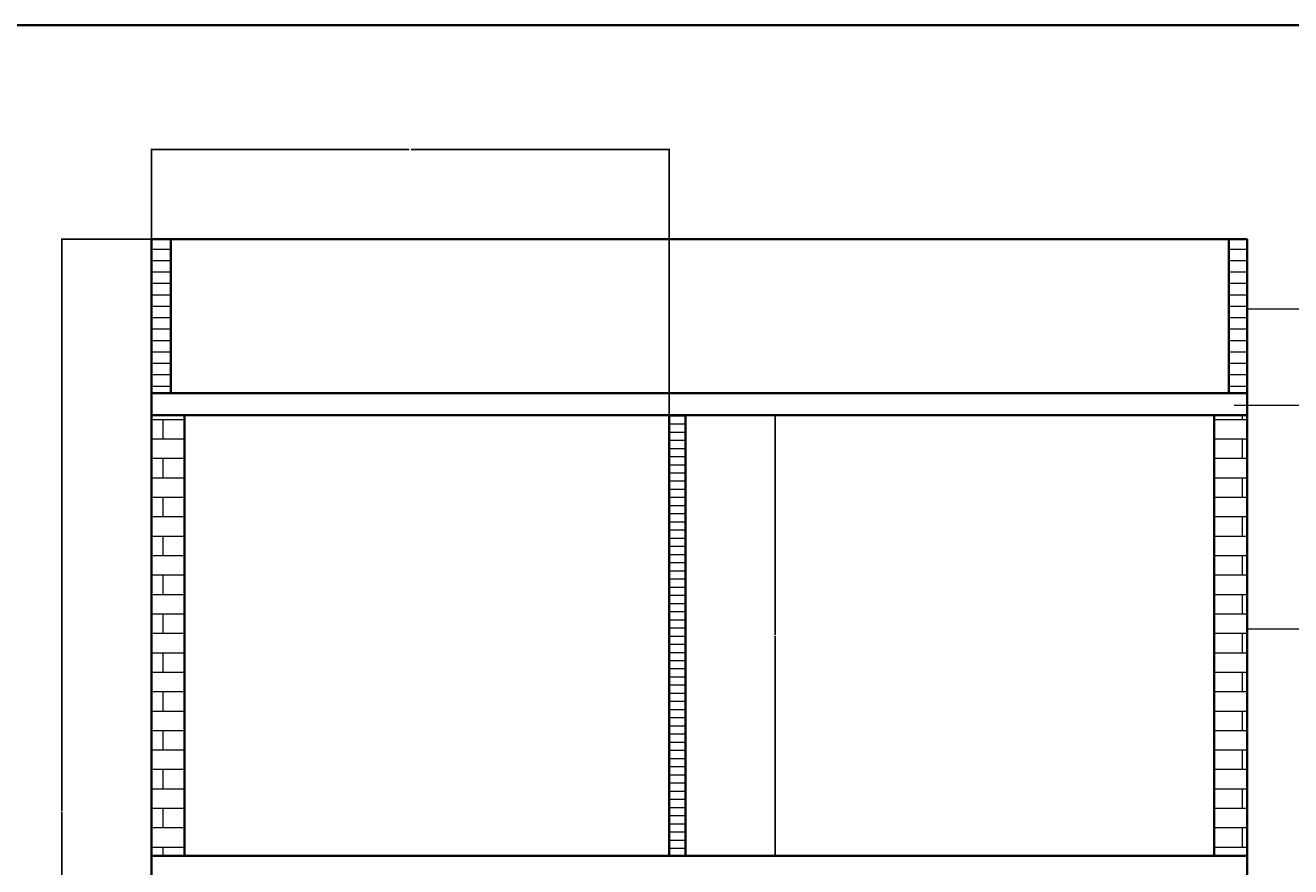
# Model space of a CAD drawing. Units: inches. Extents: x 2416 to 3391, y 1375 to 2496.
# Tile 12 of 13: x 2870 to 3215, y 2267 to 2496. Entities that reach past the tile are written whole.
import ezdxf

# ---------------------------------------------------------------- set-up
doc = ezdxf.new("R2010")
doc.units = ezdxf.units.IN
for name, color, linetype, lineweight in [('A-ANNO-DIMS', 2, 'Continuous', 18), ('A-ANNO-TEXT', 7, 'Continuous', 18), ('A-ANNO-TTLB', 7, 'Continuous', 35), ('A-SECT', 7, 'Continuous', 35), ('A-WALL-PATT', 252, 'Continuous', 13)]:
    doc.layers.add(name, color=color, linetype=linetype, lineweight=lineweight)
doc.styles.get("Standard").update_dxf_attribs({"font": 'arial.ttf'})
doc.dimstyles.get("Standard").update_dxf_attribs({"dimtxt": 0.18, "dimasz": 0.18, "dimexe": 0.18, "dimexo": 0.0625, "dimgap": 0.09, "dimtad": 0, "dimtih": 1, "dimtoh": 1, "dimdec": 4, "dimzin": 0, "dimdsep": 46, "dimtxsty": 'Standard', "dimcen": 0.09, "dimadec": 0, "dimazin": 0, "dimtfac": 1, "dimtdec": 4, "dimtofl": 0, "dimtmove": 0, "dimatfit": 3, "dimfxl": 1, "dimtolj": 1, "dimtzin": 0, "dimarcsym": 0})

# ---------------------------------------------------------------- blocks, each defined once
blk = doc.blocks.new('*D84')
at = {"layer": 'A-ANNO-DIMS', "color": 0, "lineweight": -2, "transparency": 16777216}
for p, q in [((2904.13, 2437.86), (2879.61, 2437.86)), ((2879.79, 2437.68), (2879.79, 2282.04)), ((2879.79, 2126.04), (2879.79, 2281.68)), ((2904.13, 2125.86), (2879.61, 2125.86))]:
    blk.add_line(p, q, dxfattribs=at)
at = {"layer": 'A-ANNO-DIMS', "color": 0, "transparency": 16777216}
for points in [[(2879.76, 2437.68), (2879.82, 2437.68), (2879.79, 2437.86)], [(2879.76, 2126.04), (2879.82, 2126.04), (2879.79, 2125.86)]]:
    blk.add_solid(points, dxfattribs=at)
at = {"layer": 'Defpoints', "color": 0, "transparency": 16777216}
for p in [(2879.79, 2437.86), (2904.19, 2437.86), (2904.19, 2125.86)]:
    blk.add_point(p, dxfattribs=at)
at = {"layer": 'A-ANNO-DIMS', "color": 0, "transparency": 16777216, "insert": (2879.79, 2281.86), "char_height": 0.18, "attachment_point": 5}
blk.add_mtext('\\A1;312', dxfattribs=at)
blk = doc.blocks.new('*D85')
at = {"layer": 'A-ANNO-DIMS', "color": 0, "lineweight": -2, "transparency": 16777216}
for p, q in [((2904.19, 2437.92), (2904.19, 2462.44)), ((2904.37, 2462.26), (2974.43, 2462.26)), ((3045.01, 2462.26), (2974.96, 2462.26)), ((3045.19, 2389.92), (3045.19, 2462.44))]:
    blk.add_line(p, q, dxfattribs=at)
at = {"layer": 'A-ANNO-DIMS', "color": 0, "transparency": 16777216}
for points in [[(2904.37, 2462.29), (2904.37, 2462.23), (2904.19, 2462.26)], [(3045.01, 2462.29), (3045.01, 2462.23), (3045.19, 2462.26)]]:
    blk.add_solid(points, dxfattribs=at)
at = {"layer": 'Defpoints', "color": 0, "transparency": 16777216}
for p in [(3045.19, 2462.26), (2904.19, 2437.86), (3045.19, 2389.86)]:
    blk.add_point(p, dxfattribs=at)
at = {"layer": 'A-ANNO-DIMS', "color": 0, "transparency": 16777216, "insert": (2974.69, 2462.26), "char_height": 0.18, "attachment_point": 5}
blk.add_mtext('\\A1;141', dxfattribs=at)
blk = doc.blocks.new('*D87')
at = {"layer": 'A-ANNO-DIMS', "color": 0, "lineweight": -2, "transparency": 16777216}
for p, q in [((3049.75, 2389.86), (3074.27, 2389.86)), ((3074.09, 2389.68), (3074.09, 2330.04)), ((3074.09, 2270.04), (3074.09, 2329.68)), ((3049.75, 2269.86), (3074.27, 2269.86))]:
    blk.add_line(p, q, dxfattribs=at)
at = {"layer": 'A-ANNO-DIMS', "color": 0, "transparency": 16777216}
for points in [[(3074.06, 2389.68), (3074.12, 2389.68), (3074.09, 2389.86)], [(3074.06, 2270.04), (3074.12, 2270.04), (3074.09, 2269.86)]]:
    blk.add_solid(points, dxfattribs=at)
at = {"layer": 'Defpoints', "color": 0, "transparency": 16777216}
for p in [(3049.69, 2389.86), (3049.69, 2269.86), (3074.09, 2269.86)]:
    blk.add_point(p, dxfattribs=at)
at = {"layer": 'A-ANNO-DIMS', "color": 0, "transparency": 16777216, "insert": (3074.09, 2329.86), "char_height": 0.18, "attachment_point": 5}
blk.add_mtext('\\A1;120', dxfattribs=at)

msp = doc.modelspace()

# ---------------------------------------------------------------- hatches: boundary and pattern name
at = {"layer": 'A-WALL-PATT'}
h = msp.add_hatch(dxfattribs=at)
h.set_pattern_fill('ANSI31', color=256, scale=0.979528, angle=-45, style=0)
h.paths.add_polyline_path([(2904.1924, 2395.8608), (2909.4444, 2395.8608), (2909.4444, 2437.8608), (2904.1924, 2437.8608)])
h = msp.add_hatch(dxfattribs=at)
h.set_pattern_fill('ANSI31', color=256, scale=0.979528, angle=-45, style=0)
h.paths.add_polyline_path([(3197.6594, 2395.8608), (3202.6924, 2395.8608), (3202.6924, 2437.8608), (3197.6594, 2437.8608)])
h = msp.add_hatch(dxfattribs=at)
h.set_pattern_fill('AR-BRSTD', color=256, scale=0.0781866, style=0)
h.paths.add_polyline_path([(2904.1924, 2269.8608), (2913.1924, 2269.8608), (2913.1924, 2389.8608), (2904.1924, 2389.8608)])
h = msp.add_hatch(dxfattribs=at)
h.set_pattern_fill('ANSI31', color=256, scale=0.7001575, angle=-45, style=0)
h.paths.add_polyline_path([(3045.1924, 2269.8608), (3049.6924, 2269.8608), (3049.6924, 2389.8608), (3045.1924, 2389.8608)])
h = msp.add_hatch(dxfattribs=at)
h.set_pattern_fill('AR-BRSTD', color=256, scale=0.0781866, style=0)
h.paths.add_polyline_path([(3193.6924, 2269.8608), (3202.6924, 2269.8608), (3202.6924, 2389.8608), (3193.6924, 2389.8608)])

# ---------------------------------------------------------------- linework, layer by layer
at = {"layer": 'A-ANNO-TEXT'}
for p, q in [((3202.6924, 2418.8281), (3249.1878, 2418.8281)), ((3199.1027, 2392.591), (3262.0173, 2392.591)), ((3202.6924, 2331.6911), (3251.2079, 2331.6911))]:
    msp.add_line(p, q, dxfattribs=at)
at = {"layer": 'A-ANNO-TTLB'}
msp.add_lwpolyline([(2416.4678, 2496.0939), (3391.2022, 2496.0939), (3391.2022, 1375.1104), (2416.4678, 1375.1104)], close=True, dxfattribs=at)
at = {"layer": 'A-SECT'}
for p, q in [((2904.1924, 2437.8608), (2904.1924, 2251.8608)), ((3202.6924, 2437.8608), (2904.1924, 2437.8608)), ((2909.4444, 2395.8608), (2909.4444, 2437.8608)), ((3197.6594, 2395.8608), (3197.6594, 2437.8608)), ((3202.6924, 2437.8608), (3202.6924, 2251.8608)), ((3202.6924, 2395.8608), (2904.1924, 2395.8608)), ((3202.6924, 2389.8608), (2904.1924, 2389.8608)), ((2913.1924, 2389.8608), (2913.1924, 2269.8608)), ((3045.1924, 2389.8608), (3045.1924, 2269.8608)), ((3049.6924, 2389.8608), (3049.6924, 2269.8608)), ((3193.6924, 2389.8608), (3193.6924, 2269.8608)), ((2904.1924, 2311.8608), (2904.1924, 2125.8608)), ((3202.6924, 2311.8608), (3202.6924, 2125.8608)), ((3202.6924, 2269.8608), (2904.1924, 2269.8608))]:
    msp.add_line(p, q, dxfattribs=at)

# ---------------------------------------------------------------- dimensions: what is measured, and where the dimension line sits
at = {"layer": 'A-ANNO-DIMS'}
dim = msp.add_linear_dim(base=(3045.1924, 2462.2608), p1=(2904.1924, 2437.8608), p2=(3045.1924, 2389.8608), dimstyle='Standard', override={"dimdec": 0, "dimlfac": 1, "dimrnd": 0, "dimzin": 0, "dimdsep": 46, "dimlunit": 2}, dxfattribs=at)
dim.commit()
dim.dimension.update_dxf_attribs({"geometry": '*D85', "text_midpoint": (2974.6924, 2462.2608)})
for base, p1, p2, angle, picture, middle in [((2879.7924, 2437.8608), (2904.1924, 2125.8608), (2904.1924, 2437.8608), 90, '*D84', (2879.7924, 2281.8608)), ((3074.0924, 2269.8608), (3049.6924, 2389.8608), (3049.6924, 2269.8608), 270, '*D87', (3074.0924, 2329.8608))]:
    dim = msp.add_linear_dim(base=base, p1=p1, p2=p2, angle=angle, dimstyle='Standard', override={"dimdec": 0, "dimlfac": 1, "dimrnd": 0, "dimzin": 0, "dimdsep": 46, "dimlunit": 2}, dxfattribs=at)
    dim.commit()
    dim.dimension.update_dxf_attribs({"geometry": picture, "text_midpoint": middle})

doc.saveas('drawing.dxf')
